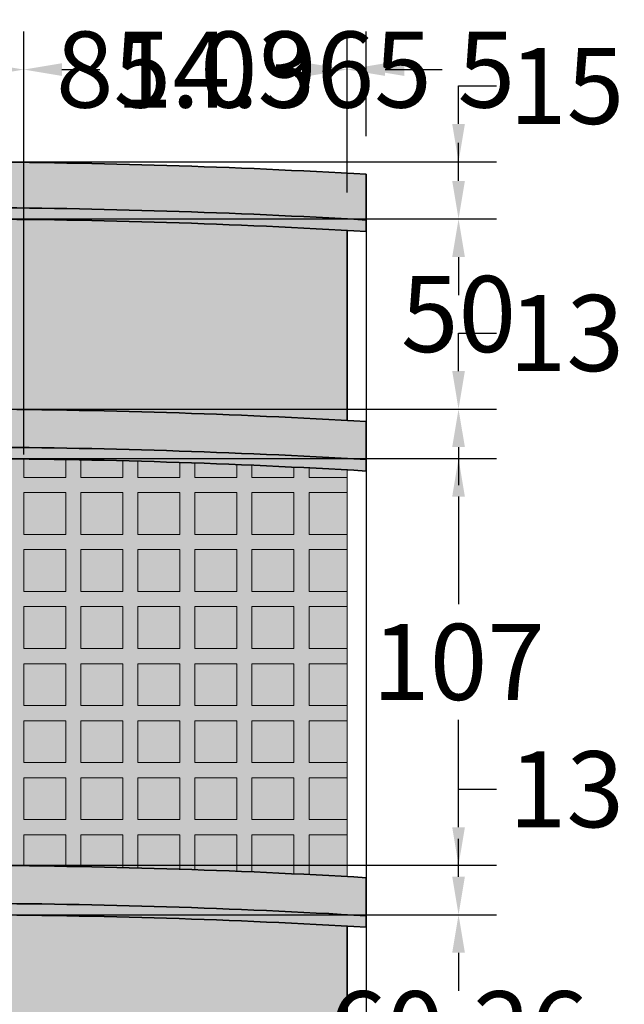
# Model space of a CAD drawing. Units: millimetres. Extents: x 130 to 1021, y 147 to 699.
# Tile 40 of 40: x 646 to 805, y 440 to 699. Entities that reach past the tile are written whole.
import ezdxf

# ---------------------------------------------------------------- set-up
doc = ezdxf.new("R2010")
doc.units = ezdxf.units.MM
doc.header["$MEASUREMENT"] = 0
for name, color, linetype, lineweight in [('A-ANNO-DIMS', 2, 'Continuous', 18), ('A-ELEV', 7, 'Continuous', 35), ('A-ELEV-PATT', 9, 'Continuous', 13), ('A-GLAZ', 4, 'Continuous', 18)]:
    doc.layers.add(name, color=color, linetype=linetype, lineweight=lineweight)
doc.styles.get("Standard").update_dxf_attribs({"font": 'arial.ttf'})
doc.dimstyles.get("Standard").update_dxf_attribs({"dimtxt": 20, "dimasz": 10, "dimexe": 10, "dimexo": 10, "dimgap": 5, "dimtad": 0, "dimtih": 1, "dimtoh": 1, "dimdec": 0, "dimzin": 0, "dimdsep": 46, "dimtxsty": 'Standard', "dimcen": 5, "dimadec": 0, "dimazin": 0, "dimtfac": 1, "dimtdec": 0, "dimtofl": 0, "dimtmove": 0, "dimatfit": 3, "dimfxl": 1, "dimtolj": 1, "dimtzin": 0, "dimarcsym": 0})

# ---------------------------------------------------------------- blocks, each defined once
blk = doc.blocks.new('GLASS-BLOCK')
for p, q in [((0, 0), (0, 11)), ((0, 11), (11, 11)), ((11, 0), (11, 11)), ((0, 0), (11, 0))]:
    blk.add_line(p, q)
blk = doc.blocks.new('*D11')
at = {"layer": 'A-ANNO-DIMS', "color": 0, "lineweight": -2, "transparency": 16777216}
for p, q in [((737.37, 648.7), (737.37, 149.74)), ((299.37, 566.95), (299.37, 149.74)), ((309.37, 159.74), (490.86, 159.74)), ((727.37, 159.74), (545.89, 159.74))]:
    blk.add_line(p, q, dxfattribs=at)
at = {"layer": 'A-ANNO-DIMS', "color": 0, "transparency": 16777216}
for points in [[(309.37, 161.41), (309.37, 158.07), (299.37, 159.74)], [(727.37, 161.41), (727.37, 158.07), (737.37, 159.74)]]:
    blk.add_solid(points, dxfattribs=at)
at = {"layer": 'Defpoints', "color": 0, "transparency": 16777216}
for p in [(737.37, 658.7), (299.37, 576.95), (737.37, 159.74)]:
    blk.add_point(p, dxfattribs=at)
at = {"layer": 'A-ANNO-DIMS', "color": 0, "transparency": 16777216, "insert": (518.37, 159.74), "char_height": 20, "attachment_point": 5}
blk.add_mtext('\\A1;438', dxfattribs=at)
blk = doc.blocks.new('*D30')
at = {"layer": 'A-ANNO-DIMS', "color": 0, "lineweight": -2, "transparency": 16777216}
for p, q in [((632.37, 593.95), (632.37, 696.25)), ((647.34, 584.98), (647.34, 696.25)), ((622.37, 686.25), (612.37, 686.25)), ((657.34, 686.25), (667.34, 686.25))]:
    blk.add_line(p, q, dxfattribs=at)
at = {"layer": 'A-ANNO-DIMS', "color": 0, "transparency": 16777216}
for points in [[(622.37, 687.91), (622.37, 684.58), (632.37, 686.25)], [(657.34, 687.91), (657.34, 684.58), (647.34, 686.25)]]:
    blk.add_solid(points, dxfattribs=at)
at = {"layer": 'Defpoints', "color": 0, "transparency": 16777216}
for p in [(647.34, 686.25), (632.37, 583.95), (647.34, 574.98)]:
    blk.add_point(p, dxfattribs=at)
at = {"layer": 'A-ANNO-DIMS', "color": 0, "transparency": 16777216, "insert": (712.99, 686.25), "char_height": 20, "attachment_point": 5}
blk.add_mtext('\\A1;14.965', dxfattribs=at)
blk = doc.blocks.new('*D31')
at = {"layer": 'A-ANNO-DIMS', "color": 0, "lineweight": -2, "transparency": 16777216}
for p, q in [((647.34, 584.98), (647.34, 696.25)), ((732.37, 653.96), (732.37, 696.25)), ((637.34, 686.25), (627.34, 686.25)), ((742.37, 686.25), (752.37, 686.25))]:
    blk.add_line(p, q, dxfattribs=at)
at = {"layer": 'A-ANNO-DIMS', "color": 0, "transparency": 16777216}
for points in [[(637.34, 687.91), (637.34, 684.58), (647.34, 686.25)], [(742.37, 687.91), (742.37, 684.58), (732.37, 686.25)]]:
    blk.add_solid(points, dxfattribs=at)
at = {"layer": 'Defpoints', "color": 0, "transparency": 16777216}
for p in [(732.37, 686.25), (732.37, 643.96), (647.34, 574.98)]:
    blk.add_point(p, dxfattribs=at)
at = {"layer": 'A-ANNO-DIMS', "color": 0, "transparency": 16777216, "insert": (689.86, 686.25), "char_height": 20, "attachment_point": 5}
blk.add_mtext('\\A1;85.03', dxfattribs=at)
blk = doc.blocks.new('*D32')
at = {"layer": 'A-ANNO-DIMS', "color": 0, "lineweight": -2, "transparency": 16777216}
for p, q in [((732.37, 653.96), (732.37, 696.25)), ((737.37, 668.7), (737.37, 696.25)), ((722.37, 686.25), (712.37, 686.25)), ((747.37, 686.25), (757.37, 686.25))]:
    blk.add_line(p, q, dxfattribs=at)
at = {"layer": 'A-ANNO-DIMS', "color": 0, "transparency": 16777216}
for points in [[(722.37, 687.91), (722.37, 684.58), (732.37, 686.25)], [(747.37, 687.91), (747.37, 684.58), (737.37, 686.25)]]:
    blk.add_solid(points, dxfattribs=at)
at = {"layer": 'Defpoints', "color": 0, "transparency": 16777216}
for p in [(737.37, 686.25), (737.37, 658.7), (732.37, 643.96)]:
    blk.add_point(p, dxfattribs=at)
at = {"layer": 'A-ANNO-DIMS', "color": 0, "transparency": 16777216, "insert": (769, 686.25), "char_height": 20, "attachment_point": 5}
blk.add_mtext('\\A1;5', dxfattribs=at)
blk = doc.blocks.new('*D54')
at = {"layer": 'A-ANNO-DIMS', "color": 0, "lineweight": -2, "transparency": 16777216}
for p, q in [((761.67, 473.95), (761.67, 483.95)), ((497.37, 463.95), (771.67, 463.95)), ((747.37, 403.69), (771.67, 403.69)), ((761.67, 393.69), (761.67, 383.69))]:
    blk.add_line(p, q, dxfattribs=at)
at = {"layer": 'A-ANNO-DIMS', "color": 0, "transparency": 16777216}
for points in [[(760.01, 473.95), (763.34, 473.95), (761.67, 463.95)], [(760.01, 393.69), (763.34, 393.69), (761.67, 403.69)]]:
    blk.add_solid(points, dxfattribs=at)
at = {"layer": 'Defpoints', "color": 0, "transparency": 16777216}
for p in [(487.37, 463.95), (761.67, 463.95), (737.37, 403.69)]:
    blk.add_point(p, dxfattribs=at)
at = {"layer": 'A-ANNO-DIMS', "color": 0, "transparency": 16777216, "insert": (761.67, 433.82), "char_height": 20, "attachment_point": 5}
blk.add_mtext('\\A1;60.26', dxfattribs=at)
blk = doc.blocks.new('*D55')
at = {"layer": 'A-ANNO-DIMS', "color": 0, "lineweight": -2, "transparency": 16777216}
for p, q in [((761.67, 486.95), (761.67, 496.95)), ((761.67, 496.95), (771.67, 496.95)), ((562.37, 476.95), (771.67, 476.95)), ((497.37, 463.95), (771.67, 463.95)), ((761.67, 453.95), (761.67, 443.95))]:
    blk.add_line(p, q, dxfattribs=at)
at = {"layer": 'A-ANNO-DIMS', "color": 0, "transparency": 16777216}
for points in [[(760.01, 486.95), (763.34, 486.95), (761.67, 476.95)], [(760.01, 453.95), (763.34, 453.95), (761.67, 463.95)]]:
    blk.add_solid(points, dxfattribs=at)
at = {"layer": 'Defpoints', "color": 0, "transparency": 16777216}
for p in [(552.37, 476.95), (761.67, 476.95), (487.37, 463.95)]:
    blk.add_point(p, dxfattribs=at)
at = {"layer": 'A-ANNO-DIMS', "color": 0, "transparency": 16777216, "insert": (790.06, 496.95), "char_height": 20, "attachment_point": 5}
blk.add_mtext('\\A1;13', dxfattribs=at)
blk = doc.blocks.new('*D56')
at = {"layer": 'A-ANNO-DIMS', "color": 0, "lineweight": -2, "transparency": 16777216}
for p, q in [((562.37, 583.95), (771.67, 583.95)), ((761.67, 573.95), (761.67, 545.66)), ((761.67, 486.95), (761.67, 515.24)), ((562.37, 476.95), (771.67, 476.95))]:
    blk.add_line(p, q, dxfattribs=at)
at = {"layer": 'A-ANNO-DIMS', "color": 0, "transparency": 16777216}
for points in [[(760.01, 573.95), (763.34, 573.95), (761.67, 583.95)], [(760.01, 486.95), (763.34, 486.95), (761.67, 476.95)]]:
    blk.add_solid(points, dxfattribs=at)
at = {"layer": 'Defpoints', "color": 0, "transparency": 16777216}
for p in [(552.37, 583.95), (761.67, 583.95), (552.37, 476.95)]:
    blk.add_point(p, dxfattribs=at)
at = {"layer": 'A-ANNO-DIMS', "color": 0, "transparency": 16777216, "insert": (761.67, 530.45), "char_height": 20, "attachment_point": 5}
blk.add_mtext('\\A1;107', dxfattribs=at)
blk = doc.blocks.new('*D57')
at = {"layer": 'A-ANNO-DIMS', "color": 0, "lineweight": -2, "transparency": 16777216}
for p, q in [((761.67, 606.95), (761.67, 616.95)), ((761.67, 616.95), (771.67, 616.95)), ((497.37, 596.95), (771.67, 596.95)), ((562.37, 583.95), (771.67, 583.95)), ((761.67, 573.95), (761.67, 563.95))]:
    blk.add_line(p, q, dxfattribs=at)
at = {"layer": 'A-ANNO-DIMS', "color": 0, "transparency": 16777216}
for points in [[(760.01, 606.95), (763.34, 606.95), (761.67, 596.95)], [(760.01, 573.95), (763.34, 573.95), (761.67, 583.95)]]:
    blk.add_solid(points, dxfattribs=at)
at = {"layer": 'Defpoints', "color": 0, "transparency": 16777216}
for p in [(487.37, 596.95), (761.67, 596.95), (552.37, 583.95)]:
    blk.add_point(p, dxfattribs=at)
at = {"layer": 'A-ANNO-DIMS', "color": 0, "transparency": 16777216, "insert": (790.06, 616.95), "char_height": 20, "attachment_point": 5}
blk.add_mtext('\\A1;13', dxfattribs=at)
blk = doc.blocks.new('*D58')
at = {"layer": 'A-ANNO-DIMS', "color": 0, "lineweight": -2, "transparency": 16777216}
for p, q in [((761.67, 656.95), (761.67, 666.95)), ((497.37, 646.95), (771.67, 646.95)), ((497.37, 596.95), (771.67, 596.95)), ((761.67, 586.95), (761.67, 576.95))]:
    blk.add_line(p, q, dxfattribs=at)
at = {"layer": 'A-ANNO-DIMS', "color": 0, "transparency": 16777216}
for points in [[(760.01, 656.95), (763.34, 656.95), (761.67, 646.95)], [(760.01, 586.95), (763.34, 586.95), (761.67, 596.95)]]:
    blk.add_solid(points, dxfattribs=at)
at = {"layer": 'Defpoints', "color": 0, "transparency": 16777216}
for p in [(487.37, 646.95), (761.67, 646.95), (487.37, 596.95)]:
    blk.add_point(p, dxfattribs=at)
at = {"layer": 'A-ANNO-DIMS', "color": 0, "transparency": 16777216, "insert": (761.67, 621.95), "char_height": 20, "attachment_point": 5}
blk.add_mtext('\\A1;50', dxfattribs=at)
blk = doc.blocks.new('*D59')
at = {"layer": 'A-ANNO-DIMS', "color": 0, "lineweight": -2, "transparency": 16777216}
for p, q in [((761.67, 671.95), (761.67, 681.95)), ((761.67, 681.95), (771.67, 681.95)), ((497.37, 661.95), (771.67, 661.95)), ((497.37, 646.95), (771.67, 646.95)), ((761.67, 636.95), (761.67, 626.95))]:
    blk.add_line(p, q, dxfattribs=at)
at = {"layer": 'A-ANNO-DIMS', "color": 0, "transparency": 16777216}
for points in [[(760.01, 671.95), (763.34, 671.95), (761.67, 661.95)], [(760.01, 636.95), (763.34, 636.95), (761.67, 646.95)]]:
    blk.add_solid(points, dxfattribs=at)
at = {"layer": 'Defpoints', "color": 0, "transparency": 16777216}
for p in [(487.37, 661.95), (761.67, 661.95), (487.37, 646.95)]:
    blk.add_point(p, dxfattribs=at)
at = {"layer": 'A-ANNO-DIMS', "color": 0, "transparency": 16777216, "insert": (790.13, 681.95), "char_height": 20, "attachment_point": 5}
blk.add_mtext('\\A1;15', dxfattribs=at)

msp = doc.modelspace()

# ---------------------------------------------------------------- hatches: boundary and pattern name
at = {"layer": 'A-ELEV-PATT'}
h = msp.add_hatch(color=256, dxfattribs=at)
h.dxf.hatch_style = 1
h.paths.add_polyline_path([(737.3738, 658.6988, 0.01359606), (632.4019, 661.9473), (607.3738, 661.9473), (487.3738, 661.9473), (487.3738, 649.9473), (607.3738, 649.9473), (632.3794, 649.9473, -0.01368411), (737.3738, 646.6784)])
h.paths.add_polyline_path([(732.3738, 643.9599, 0.01305286), (632.3738, 646.9473), (607.3738, 646.9473), (487.3738, 646.9473), (487.3738, 596.9473), (632.3738, 596.9473, -0.01305286), (732.3738, 593.9599)])
h.paths.add_polyline_path([(737.3738, 593.6732, 0.01370629), (632.3738, 596.9473), (487.3738, 596.9473), (487.3738, 586.9473), (632.355, 586.9473, -0.01378075), (737.3738, 583.6559)])
h.paths.add_polyline_path([(447.3738, 646.9473), (307.3738, 646.9473), (302.3738, 646.9473), (302.3738, 634.9473), (447.3738, 634.9473)])
h.paths.add_polyline_path([(447.3738, 631.9473), (307.3738, 631.9473), (307.3738, 586.9473), (447.3738, 586.9473)])
h.paths.add_polyline_path([(447.3738, 586.9473), (307.3738, 586.9473), (302.3738, 586.9473), (302.3738, 576.9473), (447.3738, 576.9473)])
h.paths.add_polyline_path([(447.3738, 573.9473), (367.3738, 573.9473), (367.3738, 539.9473), (447.3738, 539.9473)])
h.paths.add_polyline_path([(447.3738, 537.9473), (367.3738, 537.9473), (367.3738, 507.9473), (400.392, 507.4253, -0.00172798), (401.3281, 507.6451, -0.52200255), (425.6117, 511.0391, -0.03918489), (447.3738, 510.4359), (447.3738, 510.7883)])
h.paths.add_polyline_path([(394.7238, 505.9473), (367.3738, 505.9473), (367.3738, 476.9473, -0.0146512), (375.8501, 480.2159), (376.1506, 499.2266, -0.03554194)])
h.paths.add_polyline_path([(632.3738, 583.9473), (552.3738, 583.9473), (552.3738, 550.9473), (632.3738, 550.9473)])
h.paths.add_polyline_path([(632.3738, 548.9473), (552.3738, 548.9473), (552.3738, 515.9473), (632.3738, 515.9473)])
h.paths.add_polyline_path([(632.3738, 513.9473), (552.3738, 513.9473), (552.3738, 476.9473), (632.3738, 476.9473)])
h.paths.add_polyline_path([(737.3738, 473.6903, 0.01363261), (632.3926, 476.9473), (552.3738, 476.9473), (487.3738, 476.9473), (487.3738, 466.9473), (632.3738, 466.9473, -0.01370629), (737.3738, 463.6732)])
h.paths.add_polyline_path([(732.3738, 460.9552, 0.01307409), (632.3681, 463.9473), (487.3738, 463.9473), (487.3738, 407.735, -0.00322862), (489.3544, 406.9473), (632.3926, 406.9473, -0.01298259), (732.3738, 403.9755)])
h.paths.add_polyline_path([(487.3738, 463.9473, 0.20132998), (367.3738, 463.9473), (367.3738, 407.735, -0.18820307), (487.3738, 407.735)])
h.paths.add_polyline_path([(367.3738, 476.9473), (367.3738, 466.9473, -0.20133085), (487.3738, 466.9473), (487.3738, 476.9473, 0.20132998)])
h.paths.add_polyline_path([(367.3738, 463.9473), (307.3738, 463.9473), (307.3738, 401.9473), (357.9413, 401.9473), (367.3738, 407.735)])
h.paths.add_polyline_path([(367.3738, 476.9473), (302.3738, 476.9473), (302.3738, 466.9473), (367.3738, 466.9473)])
h.paths.add_polyline_path([(632.8184, 366.9453), (552.3738, 366.9453), (552.3738, 393.9473), (632.8184, 393.9473)])
h.paths.add_polyline_path([(632.8184, 357.2114), (632.8184, 363.9453), (552.3738, 363.9453), (552.3738, 357.2114), (552.3738, 336.9453), (632.8184, 336.9453)])
h.paths.add_polyline_path([(632.8184, 333.9453), (552.3738, 333.9453), (552.3738, 306.9453), (632.8184, 306.9453)])
h.paths.add_polyline_path([(632.8184, 303.9453), (552.3738, 303.9453), (552.3738, 273.9473), (632.355, 273.9473, 0.00006077), (632.8184, 273.9491)])
h.paths.add_polyline_path([(737.3738, 403.6903, 0.01363261), (632.3926, 406.9473), (489.3544, 406.9473, 0.19154808), (367.3738, 407.735), (367.3738, 396.9473, -0.20133085), (487.3738, 396.9473), (632.3738, 396.9473, -0.01370629), (737.3738, 393.6732)])
h.paths.add_polyline_path([(357.9413, 401.9473), (307.3738, 401.9473), (307.3738, 391.9473), (357.9413, 391.9473)])
h.paths.add_polyline_path([(357.9413, 357.2114), (357.9413, 388.9473), (307.3738, 388.9473), (307.3738, 357.2114), (307.3738, 273.9473), (357.9413, 273.9473)])
h.paths.add_polyline_path([(732.3738, 263.93, -0.0130317), (632.3794, 260.9473), (466.7667, 260.9473), (466.7667, 240.9473), (469.8406, 236.978), (469.8406, 221.978), (472.9145, 218.0087), (472.9145, 213.9473), (607.3738, 213.9473), (732.3738, 213.9473)])
h.paths.add_polyline_path([(732.3738, 290.889), (722.479, 290.889), (722.479, 301.889), (732.3738, 301.889), (732.3738, 305.889), (722.479, 305.889), (722.479, 316.889), (732.3738, 316.889), (732.3738, 320.889), (722.479, 320.889), (722.479, 331.889), (732.3738, 331.889), (732.3738, 335.889), (722.479, 335.889), (722.479, 346.889), (732.3738, 346.889), (732.3738, 350.889), (722.479, 350.889), (722.479, 361.889), (732.3738, 361.889), (732.3738, 365.889), (722.479, 365.889), (722.479, 376.889), (732.3738, 376.889), (732.3738, 380.889), (722.479, 380.889), (722.479, 391.4848, 0.00052326), (718.479, 391.6843), (718.479, 380.889), (707.479, 380.889), (707.479, 392.1896, 0.00052307), (703.479, 392.3576), (703.479, 380.889), (692.479, 380.889), (692.479, 392.7765, 0.00052292), (688.479, 392.9131), (688.479, 380.889), (677.479, 380.889), (677.479, 393.2456, 0.00052279), (673.479, 393.3508), (673.479, 380.889), (662.479, 380.889), (662.479, 393.597, 0.0005227), (658.479, 393.6709), (658.479, 380.889), (647.479, 380.889), (647.479, 393.8308, 0.00052264), (643.479, 393.8732), (643.479, 380.889), (632.8184, 380.889), (632.8184, 376.889), (643.479, 376.889), (643.479, 365.889), (632.8184, 365.889), (632.8184, 361.889), (643.479, 361.889), (643.479, 350.889), (632.8184, 350.889), (632.8184, 346.889), (643.479, 346.889), (643.479, 335.889), (632.8184, 335.889), (632.8184, 331.889), (643.479, 331.889), (643.479, 320.889), (632.8184, 320.889), (632.8184, 316.889), (643.479, 316.889), (643.479, 305.889), (632.8184, 305.889), (632.8184, 301.889), (643.479, 301.889), (643.479, 290.889), (632.8184, 290.889), (632.8184, 286.889), (643.479, 286.889), (643.479, 274.0217, 0.00052456), (647.479, 274.0643), (647.479, 286.889), (658.479, 286.889), (658.479, 274.2248, 0.00052462), (662.479, 274.2989), (662.479, 286.889), (673.479, 286.889), (673.479, 274.546, 0.00052471), (677.479, 274.6516), (677.479, 286.889), (688.479, 286.889), (688.479, 274.9853, 0.00052484), (692.479, 275.1224), (692.479, 286.889), (703.479, 286.889), (703.479, 275.5429, 0.000525), (707.479, 275.7115), (707.479, 286.889), (718.479, 286.889), (718.479, 276.2187, 0.00052519), (722.479, 276.4189), (722.479, 286.889), (732.3738, 286.889)])
h.paths.add_polyline_path([(718.479, 290.889), (707.479, 290.889), (707.479, 301.889), (718.479, 301.889)], flags=16)
h.paths.add_polyline_path([(703.479, 290.889), (692.479, 290.889), (692.479, 301.889), (703.479, 301.889)], flags=16)
h.paths.add_polyline_path([(718.479, 305.889), (707.479, 305.889), (707.479, 316.889), (718.479, 316.889)], flags=16)
h.paths.add_polyline_path([(703.479, 305.889), (692.479, 305.889), (692.479, 316.889), (703.479, 316.889)], flags=16)
h.paths.add_polyline_path([(688.479, 290.889), (677.479, 290.889), (677.479, 301.889), (688.479, 301.889)], flags=16)
h.paths.add_polyline_path([(718.479, 320.889), (707.479, 320.889), (707.479, 331.889), (718.479, 331.889)], flags=16)
h.paths.add_polyline_path([(688.479, 305.889), (677.479, 305.889), (677.479, 316.889), (688.479, 316.889)], flags=16)
h.paths.add_polyline_path([(703.479, 320.889), (692.479, 320.889), (692.479, 331.889), (703.479, 331.889)], flags=16)
h.paths.add_polyline_path([(688.479, 320.889), (677.479, 320.889), (677.479, 331.889), (688.479, 331.889)], flags=16)
h.paths.add_polyline_path([(673.479, 290.889), (662.479, 290.889), (662.479, 301.889), (673.479, 301.889)], flags=16)
h.paths.add_polyline_path([(718.479, 335.889), (707.479, 335.889), (707.479, 346.889), (718.479, 346.889)], flags=16)
h.paths.add_polyline_path([(673.479, 305.889), (662.479, 305.889), (662.479, 316.889), (673.479, 316.889)], flags=16)
h.paths.add_polyline_path([(703.479, 335.889), (692.479, 335.889), (692.479, 346.889), (703.479, 346.889)], flags=16)
h.paths.add_polyline_path([(673.479, 320.889), (662.479, 320.889), (662.479, 331.889), (673.479, 331.889)], flags=16)
h.paths.add_polyline_path([(688.479, 335.889), (677.479, 335.889), (677.479, 346.889), (688.479, 346.889)], flags=16)
h.paths.add_polyline_path([(658.479, 290.889), (647.479, 290.889), (647.479, 301.889), (658.479, 301.889)], flags=16)
h.paths.add_polyline_path([(718.479, 350.889), (707.479, 350.889), (707.479, 361.889), (718.479, 361.889)], flags=16)
h.paths.add_polyline_path([(658.479, 305.889), (647.479, 305.889), (647.479, 316.889), (658.479, 316.889)], flags=16)
h.paths.add_polyline_path([(703.479, 350.889), (692.479, 350.889), (692.479, 361.889), (703.479, 361.889)], flags=16)
h.paths.add_polyline_path([(673.479, 335.889), (662.479, 335.889), (662.479, 346.889), (673.479, 346.889)], flags=16)
h.paths.add_polyline_path([(658.479, 320.889), (647.479, 320.889), (647.479, 331.889), (658.479, 331.889)], flags=16)
h.paths.add_polyline_path([(688.479, 350.889), (677.479, 350.889), (677.479, 361.889), (688.479, 361.889)], flags=16)
h.paths.add_polyline_path([(718.479, 365.889), (707.479, 365.889), (707.479, 376.889), (718.479, 376.889)], flags=16)
h.paths.add_polyline_path([(658.479, 335.889), (647.479, 335.889), (647.479, 346.889), (658.479, 346.889)], flags=16)
h.paths.add_polyline_path([(673.479, 350.889), (662.479, 350.889), (662.479, 361.889), (673.479, 361.889)], flags=16)
h.paths.add_polyline_path([(703.479, 365.889), (692.479, 365.889), (692.479, 376.889), (703.479, 376.889)], flags=16)
h.paths.add_polyline_path([(688.479, 365.889), (677.479, 365.889), (677.479, 376.889), (688.479, 376.889)], flags=16)
h.paths.add_polyline_path([(658.479, 350.889), (647.479, 350.889), (647.479, 361.889), (658.479, 361.889)], flags=16)
h.paths.add_polyline_path([(673.479, 365.889), (662.479, 365.889), (662.479, 376.889), (673.479, 376.889)], flags=16)
h.paths.add_polyline_path([(658.479, 365.889), (647.479, 365.889), (647.479, 376.889), (658.479, 376.889)], flags=16)
h.paths.add_polyline_path([(732.3738, 503.9786), (722.3392, 503.9786), (722.3392, 514.9786), (732.3738, 514.9786), (732.3738, 518.9786), (722.3392, 518.9786), (722.3392, 529.9786), (732.3738, 529.9786), (732.3738, 533.9786), (722.3392, 533.9786), (722.3392, 544.9786), (732.3738, 544.9786), (732.3738, 546.9473), (732.3738, 548.9786), (722.3392, 548.9786), (722.3392, 559.9786), (732.3738, 559.9786), (732.3738, 563.9786), (722.3392, 563.9786), (722.3392, 574.9786), (732.3738, 574.9786), (732.3738, 578.9786), (722.3392, 578.9786), (722.3392, 581.4789, 0.00052601), (718.3392, 581.6791), (718.3392, 578.9786), (707.3392, 578.9786), (707.3392, 582.1863, 0.00052582), (703.3392, 582.355), (703.3392, 578.9786), (692.3392, 578.9786), (692.3392, 582.7752, 0.00052566), (688.3392, 582.9123), (688.3392, 578.9786), (677.3392, 578.9786), (677.3392, 583.2457, 0.00052554), (673.3392, 583.3512), (673.3392, 578.9786), (662.3392, 578.9786), (662.3392, 583.5978, 0.00052545), (658.3392, 583.6718), (658.3392, 578.9786), (647.3392, 578.9786), (647.3392, 583.8317, 0.00052539), (643.3392, 583.8741), (643.3392, 578.9786), (632.3738, 578.9786), (632.3738, 574.9786), (643.3392, 574.9786), (643.3392, 563.9786), (632.3738, 563.9786), (632.3738, 559.9786), (643.3392, 559.9786), (643.3392, 548.9786), (632.3738, 548.9786), (632.3738, 544.9786), (643.3392, 544.9786), (643.3392, 533.9786), (632.3738, 533.9786), (632.3738, 529.9786), (643.3392, 529.9786), (643.3392, 518.9786), (632.3738, 518.9786), (632.3738, 515.9473), (632.3738, 514.9786), (643.3392, 514.9786), (643.3392, 503.9786), (632.3738, 503.9786), (632.3738, 499.9786), (643.3392, 499.9786), (643.3392, 488.9786), (632.3738, 488.9786), (632.3738, 484.9786), (643.3392, 484.9786), (643.3392, 476.8751, -0.00051911), (647.3392, 476.8332), (647.3392, 484.9786), (658.3392, 484.9786), (658.3392, 476.6752, -0.00051917), (662.3392, 476.6022), (662.3392, 484.9786), (673.3392, 484.9786), (673.3392, 476.3585, -0.00051926), (677.3392, 476.2543), (677.3392, 484.9786), (688.3392, 484.9786), (688.3392, 475.9248, -0.00051938), (692.3392, 475.7894), (692.3392, 484.9786), (703.3392, 484.9786), (703.3392, 475.3741, -0.00051953), (707.3392, 475.2075), (707.3392, 484.9786), (718.3392, 484.9786), (718.3392, 474.7064, -0.00051972), (722.3392, 474.5086), (722.3392, 484.9786), (732.3738, 484.9786), (732.3738, 488.9786), (722.3392, 488.9786), (722.3392, 499.9786), (732.3738, 499.9786)])
h.paths.add_polyline_path([(718.3392, 503.9786), (707.3392, 503.9786), (707.3392, 514.9786), (718.3392, 514.9786)], flags=16)
h.paths.add_polyline_path([(718.3392, 499.9786), (718.3392, 488.9786), (707.3392, 488.9786), (707.3392, 499.9786)], flags=16)
h.paths.add_polyline_path([(718.3392, 518.9786), (707.3392, 518.9786), (707.3392, 529.9786), (718.3392, 529.9786)], flags=16)
h.paths.add_polyline_path([(703.3392, 503.9786), (692.3392, 503.9786), (692.3392, 514.9786), (703.3392, 514.9786)], flags=16)
h.paths.add_polyline_path([(703.3392, 499.9786), (703.3392, 488.9786), (692.3392, 488.9786), (692.3392, 499.9786)], flags=16)
h.paths.add_polyline_path([(703.3392, 518.9786), (692.3392, 518.9786), (692.3392, 529.9786), (703.3392, 529.9786)], flags=16)
h.paths.add_polyline_path([(718.3392, 533.9786), (707.3392, 533.9786), (707.3392, 544.9786), (718.3392, 544.9786)], flags=16)
h.paths.add_polyline_path([(688.3392, 503.9786), (677.3392, 503.9786), (677.3392, 514.9786), (688.3392, 514.9786)], flags=16)
h.paths.add_polyline_path([(688.3392, 499.9786), (688.3392, 488.9786), (677.3392, 488.9786), (677.3392, 499.9786)], flags=16)
h.paths.add_polyline_path([(703.3392, 533.9786), (692.3392, 533.9786), (692.3392, 544.9786), (703.3392, 544.9786)], flags=16)
h.paths.add_polyline_path([(688.3392, 518.9786), (677.3392, 518.9786), (677.3392, 529.9786), (688.3392, 529.9786)], flags=16)
h.paths.add_polyline_path([(688.3392, 533.9786), (677.3392, 533.9786), (677.3392, 544.9786), (688.3392, 544.9786)], flags=16)
h.paths.add_polyline_path([(718.3392, 548.9786), (707.3392, 548.9786), (707.3392, 559.9786), (718.3392, 559.9786)], flags=16)
h.paths.add_polyline_path([(673.3392, 503.9786), (662.3392, 503.9786), (662.3392, 514.9786), (673.3392, 514.9786)], flags=16)
h.paths.add_polyline_path([(673.3392, 499.9786), (673.3392, 488.9786), (662.3392, 488.9786), (662.3392, 499.9786)], flags=16)
h.paths.add_polyline_path([(703.3392, 548.9786), (692.3392, 548.9786), (692.3392, 559.9786), (703.3392, 559.9786)], flags=16)
h.paths.add_polyline_path([(673.3392, 518.9786), (662.3392, 518.9786), (662.3392, 529.9786), (673.3392, 529.9786)], flags=16)
h.paths.add_polyline_path([(688.3392, 548.9786), (677.3392, 548.9786), (677.3392, 559.9786), (688.3392, 559.9786)], flags=16)
h.paths.add_polyline_path([(673.3392, 533.9786), (662.3392, 533.9786), (662.3392, 544.9786), (673.3392, 544.9786)], flags=16)
h.paths.add_polyline_path([(718.3392, 563.9786), (707.3392, 563.9786), (707.3392, 574.9786), (718.3392, 574.9786)], flags=16)
h.paths.add_polyline_path([(658.3392, 503.9786), (647.3392, 503.9786), (647.3392, 514.9786), (658.3392, 514.9786)], flags=16)
h.paths.add_polyline_path([(658.3392, 499.9786), (658.3392, 488.9786), (647.3392, 488.9786), (647.3392, 499.9786)], flags=16)
h.paths.add_polyline_path([(703.3392, 563.9786), (692.3392, 563.9786), (692.3392, 574.9786), (703.3392, 574.9786)], flags=16)
h.paths.add_polyline_path([(658.3392, 518.9786), (647.3392, 518.9786), (647.3392, 529.9786), (658.3392, 529.9786)], flags=16)
h.paths.add_polyline_path([(673.3392, 548.9786), (662.3392, 548.9786), (662.3392, 559.9786), (673.3392, 559.9786)], flags=16)
h.paths.add_polyline_path([(688.3392, 563.9786), (677.3392, 563.9786), (677.3392, 574.9786), (688.3392, 574.9786)], flags=16)
h.paths.add_polyline_path([(658.3392, 533.9786), (647.3392, 533.9786), (647.3392, 544.9786), (658.3392, 544.9786)], flags=16)
h.paths.add_polyline_path([(673.3392, 563.9786), (662.3392, 563.9786), (662.3392, 574.9786), (673.3392, 574.9786)], flags=16)
h.paths.add_polyline_path([(658.3392, 548.9786), (647.3392, 548.9786), (647.3392, 559.9786), (658.3392, 559.9786)], flags=16)
h.paths.add_polyline_path([(658.3392, 563.9786), (647.3392, 563.9786), (647.3392, 574.9786), (658.3392, 574.9786)], flags=16)
h = msp.add_hatch(color=256, dxfattribs=at)
h.dxf.hatch_style = 1
h.paths.add_polyline_path([(447.3738, 634.9473), (302.3738, 634.9473), (302.3738, 631.9473), (307.3738, 631.9473), (447.3738, 631.9473)])
h.paths.add_polyline_path([(487.3738, 646.9473), (487.3738, 649.9473), (447.3738, 634.9473), (447.3738, 631.9473)])
h.paths.add_polyline_path([(632.3794, 649.9473), (607.3738, 649.9473), (487.3738, 649.9473), (487.3738, 646.9473), (607.3738, 646.9473), (632.3738, 646.9473, -0.01370629), (737.3738, 643.6732), (737.3738, 646.6784, 0.01368411)])
h = msp.add_hatch(color=256, dxfattribs=at)
h.dxf.hatch_style = 1
h.paths.add_polyline_path([(447.3738, 576.9473), (302.3738, 576.9473), (302.3738, 573.9473), (447.3738, 573.9473)])
h.paths.add_polyline_path([(487.3738, 583.9473), (487.3738, 586.9473), (447.3738, 576.9473), (447.3738, 573.9473)])
h.paths.add_polyline_path([(632.355, 586.9473), (487.3738, 586.9473), (487.3738, 583.9473), (632.3738, 583.9473), (632.3738, 583.9472, -0.01380003), (737.3738, 580.6507), (737.3738, 583.6559, 0.01378075)])
h.paths.add_polyline_path([(367.3738, 466.9473), (302.3738, 466.9473), (302.3738, 463.9473), (367.3738, 463.9473)])
h.paths.add_polyline_path([(487.3738, 463.9473), (487.3738, 466.9473, 0.20133085), (367.3738, 466.9473), (367.3738, 463.9473, -0.20132998)])
h.paths.add_polyline_path([(632.3738, 466.9473), (487.3738, 466.9473), (487.3738, 463.9473), (632.3681, 463.9473, -0.01372855), (737.3738, 460.6681), (737.3738, 463.6732, 0.01370629)])
h.paths.add_polyline_path([(632.3738, 396.9473), (487.3738, 396.9473, 0.20133085), (367.3738, 396.9473), (367.3738, 393.9473, -0.20237172), (486.7667, 393.9473), (632.3681, 393.9473, -0.01372855), (737.3738, 390.6681), (737.3738, 393.6732, 0.01370629)])
h.paths.add_polyline_path([(357.9413, 391.9473), (307.3738, 391.9473), (307.3738, 388.9473), (357.9413, 388.9473)])
h.paths.add_polyline_path([(367.3738, 393.9473), (367.3738, 396.9473), (357.9413, 391.924), (357.9413, 388.9473), (358.058, 388.9473)])
h.paths.add_polyline_path([(737.3738, 264.2162), (737.3738, 267.2214, -0.01370629), (632.3738, 263.9473), (463.7667, 263.9473), (466.7667, 260.9473), (632.3794, 260.9473, 0.01368411)])
h.paths.add_polyline_path([(463.7667, 263.9473), (447.3738, 263.9473), (450.3738, 260.9473), (466.7667, 260.9473)])
h.paths.add_polyline_path([(447.3738, 263.9473), (432.3738, 263.9473), (432.3738, 260.9473), (450.3738, 260.9473)])
h.paths.add_polyline_path([(382.3738, 263.9473), (357.9413, 263.9473), (357.9413, 260.9473), (382.3738, 260.9473)])
h.paths.add_polyline_path([(357.9413, 263.9473), (307.3738, 263.9473), (307.3738, 260.9473), (357.9413, 260.9473)])
h = msp.add_hatch(color=256, dxfattribs=at)
h.set_gradient(color1=(122, 175, 223), color2=(76, 153, 95))
h.paths.add_polyline_path([(632.3738, 484.9786), (632.3738, 476.9474, -0.00142303), (643.3392, 476.8751), (643.3392, 484.9786)])
h.paths.add_polyline_path([(647.3392, 476.8332, -0.00142763), (658.3392, 476.6752), (658.3392, 484.9786), (647.3392, 484.9786)])
h.paths.add_polyline_path([(673.3392, 484.9786), (662.3392, 484.9786), (662.3392, 476.6022, -0.00142783), (673.3392, 476.3585)])
h.paths.add_polyline_path([(688.3392, 475.9248), (688.3392, 484.9786), (677.3392, 484.9786), (677.3392, 476.2543, -0.00142812)])
h.paths.add_polyline_path([(692.3392, 475.7894, -0.0014285), (703.3392, 475.3741), (703.3392, 484.9786), (692.3392, 484.9786)])
h.paths.add_polyline_path([(718.3392, 474.7064), (718.3392, 484.9786), (707.3392, 484.9786), (707.3392, 475.2075, -0.00142897)])
h.paths.add_polyline_path([(722.3392, 474.5086, -0.00130403), (732.3738, 473.9755), (732.3738, 484.9786), (722.3392, 484.9786)])
h.paths.add_polyline_path([(722.3392, 488.9786), (732.3738, 488.9786), (732.3738, 499.9786), (722.3392, 499.9786)])
h.paths.add_polyline_path([(707.3392, 499.9786), (707.3392, 488.9786), (718.3392, 488.9786), (718.3392, 499.9786)])
h.paths.add_polyline_path([(703.3392, 499.9786), (692.3392, 499.9786), (692.3392, 488.9786), (703.3392, 488.9786)])
h.paths.add_polyline_path([(688.3392, 499.9786), (677.3392, 499.9786), (677.3392, 488.9786), (688.3392, 488.9786)])
h.paths.add_polyline_path([(673.3392, 499.9786), (662.3392, 499.9786), (662.3392, 488.9786), (673.3392, 488.9786)])
h.paths.add_polyline_path([(658.3392, 499.9786), (647.3392, 499.9786), (647.3392, 488.9786), (658.3392, 488.9786)])
h.paths.add_polyline_path([(643.3392, 499.9786), (632.3738, 499.9786), (632.3738, 488.9786), (643.3392, 488.9786)])
h.paths.add_polyline_path([(643.3392, 514.9786), (632.3738, 514.9786), (632.3738, 503.9786), (643.3392, 503.9786)])
h.paths.add_polyline_path([(647.3392, 503.9786), (658.3392, 503.9786), (658.3392, 514.9786), (647.3392, 514.9786)])
h.paths.add_polyline_path([(673.3392, 514.9786), (662.3392, 514.9786), (662.3392, 503.9786), (673.3392, 503.9786)])
h.paths.add_polyline_path([(688.3392, 503.9786), (688.3392, 514.9786), (677.3392, 514.9786), (677.3392, 503.9786)])
h.paths.add_polyline_path([(692.3392, 503.9786), (703.3392, 503.9786), (703.3392, 514.9786), (692.3392, 514.9786)])
h.paths.add_polyline_path([(718.3392, 503.9786), (718.3392, 514.9786), (707.3392, 514.9786), (707.3392, 503.9786)])
h.paths.add_polyline_path([(732.3738, 503.9786), (732.3738, 514.9786), (722.3392, 514.9786), (722.3392, 503.9786)])
h.paths.add_polyline_path([(732.3738, 529.9786), (722.3392, 529.9786), (722.3392, 518.9786), (732.3738, 518.9786)])
h.paths.add_polyline_path([(707.3392, 518.9786), (718.3392, 518.9786), (718.3392, 529.9786), (707.3392, 529.9786)])
h.paths.add_polyline_path([(692.3392, 518.9786), (703.3392, 518.9786), (703.3392, 529.9786), (692.3392, 529.9786)])
h.paths.add_polyline_path([(688.3392, 529.9786), (677.3392, 529.9786), (677.3392, 518.9786), (688.3392, 518.9786)])
h.paths.add_polyline_path([(673.3392, 518.9786), (673.3392, 529.9786), (662.3392, 529.9786), (662.3392, 518.9786)])
h.paths.add_polyline_path([(658.3392, 529.9786), (647.3392, 529.9786), (647.3392, 518.9786), (658.3392, 518.9786)])
h.paths.add_polyline_path([(632.3738, 529.9786), (632.3738, 518.9786), (643.3392, 518.9786), (643.3392, 529.9786)])
h.paths.add_polyline_path([(643.3392, 533.9786), (643.3392, 544.9786), (632.3738, 544.9786), (632.3738, 533.9786)])
h.paths.add_polyline_path([(647.3392, 533.9786), (658.3392, 533.9786), (658.3392, 544.9786), (647.3392, 544.9786)])
h.paths.add_polyline_path([(662.3392, 533.9786), (673.3392, 533.9786), (673.3392, 544.9786), (662.3392, 544.9786)])
h.paths.add_polyline_path([(677.3392, 533.9786), (688.3392, 533.9786), (688.3392, 544.9786), (677.3392, 544.9786)])
h.paths.add_polyline_path([(692.3392, 533.9786), (703.3392, 533.9786), (703.3392, 544.9786), (692.3392, 544.9786)])
h.paths.add_polyline_path([(707.3392, 533.9786), (718.3392, 533.9786), (718.3392, 544.9786), (707.3392, 544.9786)])
h.paths.add_polyline_path([(722.3392, 533.9786), (732.3738, 533.9786), (732.3738, 544.9786), (722.3392, 544.9786)])
h.paths.add_polyline_path([(632.3738, 559.9786), (632.3738, 548.9786), (643.3392, 548.9786), (643.3392, 559.9786)])
h.paths.add_polyline_path([(632.3738, 574.9786), (632.3738, 563.9786), (643.3392, 563.9786), (643.3392, 574.9786)])
h.paths.add_polyline_path([(632.3738, 583.9472), (632.3738, 578.9786), (643.3392, 578.9786), (643.3392, 583.8741, 0.00144023)])
h.paths.add_polyline_path([(647.3392, 583.8317), (647.3392, 578.9786), (658.3392, 578.9786), (658.3392, 583.6718, 0.00144489)])
h.paths.add_polyline_path([(647.3392, 574.9786), (647.3392, 563.9786), (658.3392, 563.9786), (658.3392, 574.9786)])
h.paths.add_polyline_path([(647.3392, 559.9786), (647.3392, 548.9786), (658.3392, 548.9786), (658.3392, 559.9786)])
h.paths.add_polyline_path([(662.3392, 559.9786), (662.3392, 548.9786), (673.3392, 548.9786), (673.3392, 559.9786)])
h.paths.add_polyline_path([(673.3392, 574.9786), (662.3392, 574.9786), (662.3392, 563.9786), (673.3392, 563.9786)])
h.paths.add_polyline_path([(662.3392, 583.5978), (662.3392, 578.9786), (673.3392, 578.9786), (673.3392, 583.3512, 0.0014451)])
h.paths.add_polyline_path([(688.3392, 578.9786), (688.3392, 582.9123, 0.0014454), (677.3392, 583.2457), (677.3392, 578.9786)])
h.paths.add_polyline_path([(677.3392, 574.9786), (677.3392, 563.9786), (688.3392, 563.9786), (688.3392, 574.9786)])
h.paths.add_polyline_path([(677.3392, 559.9786), (677.3392, 548.9786), (688.3392, 548.9786), (688.3392, 559.9786)])
h.paths.add_polyline_path([(703.3392, 559.9786), (692.3392, 559.9786), (692.3392, 548.9786), (703.3392, 548.9786)])
h.paths.add_polyline_path([(707.3392, 548.9786), (718.3392, 548.9786), (718.3392, 559.9786), (707.3392, 559.9786)])
h.paths.add_polyline_path([(722.3392, 548.9786), (732.3738, 548.9786), (732.3738, 559.9786), (722.3392, 559.9786)])
h.paths.add_polyline_path([(732.3738, 563.9786), (732.3738, 574.9786), (722.3392, 574.9786), (722.3392, 563.9786)])
h.paths.add_polyline_path([(707.3392, 563.9786), (718.3392, 563.9786), (718.3392, 574.9786), (707.3392, 574.9786)])
h.paths.add_polyline_path([(692.3392, 563.9786), (703.3392, 563.9786), (703.3392, 574.9786), (692.3392, 574.9786)])
h.paths.add_polyline_path([(703.3392, 578.9786), (703.3392, 582.355, 0.00144579), (692.3392, 582.7752), (692.3392, 578.9786)])
h.paths.add_polyline_path([(718.3392, 581.6791, 0.00144627), (707.3392, 582.1863), (707.3392, 578.9786), (718.3392, 578.9786)])
h.paths.add_polyline_path([(732.3738, 578.9786), (732.3738, 580.9394, 0.00131983), (722.3392, 581.4789), (722.3392, 578.9786)])

# ---------------------------------------------------------------- linework, layer by layer
at = {"layer": 'A-ELEV'}
for p, q in [((737.3738, 643.6732), (737.3738, 658.6988)), ((732.3738, 643.9599), (732.3738, 593.9599)), ((737.3738, 593.6732), (737.3738, 580.6507)), ((737.3738, 473.6903), (737.3738, 460.6681)), ((732.3738, 403.9755), (732.3738, 460.9552))]:
    msp.add_line(p, q, dxfattribs=at)
for centre, radius, start in [((625.1665, -1269.5089), 1931.4697, 86.6695688), ((625.1665, -1269.5089), 1919.4697, 86.6487242), ((625.1665, -1269.5089), 1916.4697, 86.6434721), ((625.1665, -1319.5089), 1916.4697, 86.6434721), ((625.1665, -1319.5089), 1906.4697, 86.6258458), ((625.1665, -1319.5089), 1903.4697, 86.6205218), ((625.1665, -1449.5089), 1926.4697, 86.6609152), ((625.1665, -1449.5089), 1916.4697, 86.6434721), ((625.1665, -1449.5089), 1913.4697, 86.6382036)]:
    msp.add_arc(centre, radius, start, 89.784526, dxfattribs=at)
at = {"layer": 'A-GLAZ'}
for p, q in [((647.3392, 578.9786), (647.3392, 583.8317)), ((658.3392, 578.9786), (658.3392, 583.6718)), ((662.3392, 578.9786), (662.3392, 583.5978)), ((673.3392, 578.9786), (673.3392, 583.3512)), ((677.3392, 578.9786), (677.3392, 583.2457)), ((688.3392, 578.9786), (688.3392, 582.9123)), ((692.3392, 578.9786), (692.3392, 582.7752)), ((703.3392, 578.9786), (703.3392, 582.355)), ((707.3392, 578.9786), (707.3392, 582.1863)), ((718.3392, 578.9786), (718.3392, 581.6791)), ((722.3392, 578.9786), (722.3392, 581.4789)), ((732.3738, 580.9394), (732.3738, 546.9473)), ((647.3392, 578.9786), (658.3392, 578.9786)), ((662.3392, 578.9786), (673.3392, 578.9786)), ((677.3392, 578.9786), (688.3392, 578.9786)), ((692.3392, 578.9786), (703.3392, 578.9786)), ((707.3392, 578.9786), (718.3392, 578.9786)), ((722.3392, 578.9786), (732.3738, 578.9786)), ((722.3392, 563.9786), (722.3392, 574.9786)), ((722.3392, 574.9786), (732.3738, 574.9786)), ((722.3392, 563.9786), (732.3738, 563.9786)), ((722.3392, 548.9786), (722.3392, 559.9786)), ((722.3392, 559.9786), (732.3738, 559.9786)), ((722.3392, 548.9786), (732.3738, 548.9786)), ((732.3738, 473.9755), (732.3738, 546.9473)), ((722.3392, 533.9786), (722.3392, 544.9786)), ((722.3392, 544.9786), (732.3738, 544.9786)), ((722.3392, 533.9786), (732.3738, 533.9786)), ((722.3392, 518.9786), (722.3392, 529.9786)), ((722.3392, 529.9786), (732.3738, 529.9786)), ((722.3392, 518.9786), (732.3738, 518.9786)), ((722.3392, 503.9786), (722.3392, 514.9786)), ((722.3392, 514.9786), (732.3738, 514.9786)), ((722.3392, 503.9786), (732.3738, 503.9786)), ((722.3392, 488.9786), (722.3392, 499.9786)), ((722.3392, 499.9786), (732.3738, 499.9786)), ((722.3392, 488.9786), (732.3738, 488.9786)), ((647.3392, 476.8332), (647.3392, 484.9786)), ((647.3392, 484.9786), (658.3392, 484.9786)), ((658.3392, 476.6752), (658.3392, 484.9786)), ((662.3392, 476.6022), (662.3392, 484.9786)), ((662.3392, 484.9786), (673.3392, 484.9786)), ((673.3392, 476.3585), (673.3392, 484.9786)), ((677.3392, 476.2543), (677.3392, 484.9786)), ((677.3392, 484.9786), (688.3392, 484.9786)), ((688.3392, 475.9248), (688.3392, 484.9786)), ((692.3392, 475.7894), (692.3392, 484.9786)), ((692.3392, 484.9786), (703.3392, 484.9786)), ((703.3392, 475.3741), (703.3392, 484.9786)), ((707.3392, 475.2075), (707.3392, 484.9786)), ((707.3392, 484.9786), (718.3392, 484.9786)), ((718.3392, 474.7064), (718.3392, 484.9786)), ((722.3392, 474.5086), (722.3392, 484.9786)), ((722.3392, 484.9786), (732.3738, 484.9786))]:
    msp.add_line(p, q, dxfattribs=at)

# ---------------------------------------------------------------- block references
for p, rotation in [((658.3393, 563.9786), 89.9999999999994), ((673.3393, 563.9786), 90.00000000000063), ((688.3393, 563.9786), 90.00000000000003), ((703.3393, 563.9786), 90.00000000000003), ((718.3393, 563.9786), 89.9999999999994), ((658.3393, 548.9786), 89.9999999999994), ((673.3393, 548.9786), 90.00000000000124), ((688.3393, 548.9786), 90.00000000000063), ((703.3393, 548.9786), 90.00000000000003), ((718.3393, 548.9786), 90.00000000000003), ((658.3393, 533.9786), 90.00000000000003), ((673.3393, 533.9786), 90.00000000000124), ((688.3393, 533.9786), 90.00000000000063), ((703.3393, 533.9786), 90.00000000000063), ((718.3393, 533.9786), 89.9999999999994), ((658.3393, 518.9786), 89.99999999999883), ((673.3393, 518.9786), 89.9999999999994), ((688.3393, 518.9786), 89.9999999999994), ((703.3393, 518.9786), 89.99999999999883), ((718.3393, 518.9786), 89.9999999999994), ((658.3393, 503.9786), 89.9999999999994), ((673.3393, 503.9786), 90.00000000000063), ((688.3393, 503.9786), 89.9999999999994), ((703.3393, 503.9786), 89.99999999999883), ((718.3393, 503.9786), 89.99999999999883), ((658.3393, 488.9786), 89.99999999999883), ((673.3393, 488.9786), 90.00000000000003), ((688.3393, 488.9786), 89.99999999999883), ((703.3393, 488.9786), 90.00000000000003), ((718.3393, 488.9786), 89.9999999999994)]:
    msp.add_blockref('GLASS-BLOCK', p, dxfattribs=dict(at, rotation=rotation))

# ---------------------------------------------------------------- dimensions: what is measured, and where the dimension line sits
at = {"layer": 'A-ANNO-DIMS'}
for base, p1, p2, override, picture, middle in [((647.3392, 686.2473), (632.3738, 583.9473), (647.3392, 574.9786), {"dimdec": 3, "dimlfac": 1, "dimrnd": 0, "dimzin": 0, "dimdsep": 46, "dimlunit": 2}, '*D30', (712.9873, 686.2473)), ((732.3738, 686.2473), (647.3392, 574.9786), (732.3738, 643.9599), {"dimdec": 2, "dimlfac": 1, "dimrnd": 0, "dimzin": 0, "dimdsep": 46, "dimlunit": 2}, '*D31', (689.8565, 686.2473)), ((737.3738, 686.2473), (732.3738, 643.9599), (737.3738, 658.6988), {"dimdec": 0, "dimlfac": 1, "dimrnd": 0, "dimzin": 0, "dimdsep": 46, "dimlunit": 2}, '*D32', (769.0041, 686.2473)), ((737.3738, 159.7395), (299.3738, 576.9473), (737.3738, 658.6988), {"dimdec": 0, "dimlfac": 1, "dimrnd": 0, "dimzin": 0, "dimdsep": 46, "dimlunit": 2}, '*D11', (518.3738, 159.7395))]:
    dim = msp.add_linear_dim(base=base, p1=p1, p2=p2, dimstyle='Standard', override=override, dxfattribs=at)
    dim.commit()
    dim.dimension.update_dxf_attribs({"geometry": picture, "text_midpoint": middle})
for base, p1, p2, override, picture, middle in [((761.6738, 661.9473), (487.3738, 646.9473), (487.3738, 661.9473), {"dimdec": 0, "dimlfac": 1, "dimrnd": 0, "dimzin": 0, "dimdsep": 46, "dimlunit": 2}, '*D59', (790.1322, 681.9473)), ((761.6738, 646.9473), (487.3738, 596.9473), (487.3738, 646.9473), {"dimdec": 0, "dimlfac": 1, "dimrnd": 0, "dimzin": 0, "dimdsep": 46, "dimlunit": 2}, '*D58', (761.6738, 621.9473)), ((761.6738, 596.9473), (552.3738, 583.9473), (487.3738, 596.9473), {"dimdec": 0, "dimlfac": 1, "dimrnd": 0, "dimzin": 0, "dimdsep": 46, "dimlunit": 2}, '*D57', (790.0571, 616.9473)), ((761.6738, 583.9473), (552.3738, 476.9473), (552.3738, 583.9473), {"dimdec": 0, "dimlfac": 1, "dimrnd": 0, "dimzin": 0, "dimdsep": 46, "dimlunit": 2}, '*D56', (761.6738, 530.4473)), ((761.6738, 476.9473), (487.3738, 463.9473), (552.3738, 476.9473), {"dimdec": 0, "dimlfac": 1, "dimrnd": 0, "dimzin": 0, "dimdsep": 46, "dimlunit": 2}, '*D55', (790.0571, 496.9473)), ((761.6738, 463.9473), (737.3738, 403.6903), (487.3738, 463.9473), {"dimdec": 2, "dimlfac": 1, "dimrnd": 0, "dimzin": 0, "dimdsep": 46, "dimlunit": 2}, '*D54', (761.6738, 433.8188))]:
    dim = msp.add_linear_dim(base=base, p1=p1, p2=p2, angle=90, dimstyle='Standard', override=override, dxfattribs=at)
    dim.commit()
    dim.dimension.update_dxf_attribs({"geometry": picture, "text_midpoint": middle})

doc.saveas('drawing.dxf')
